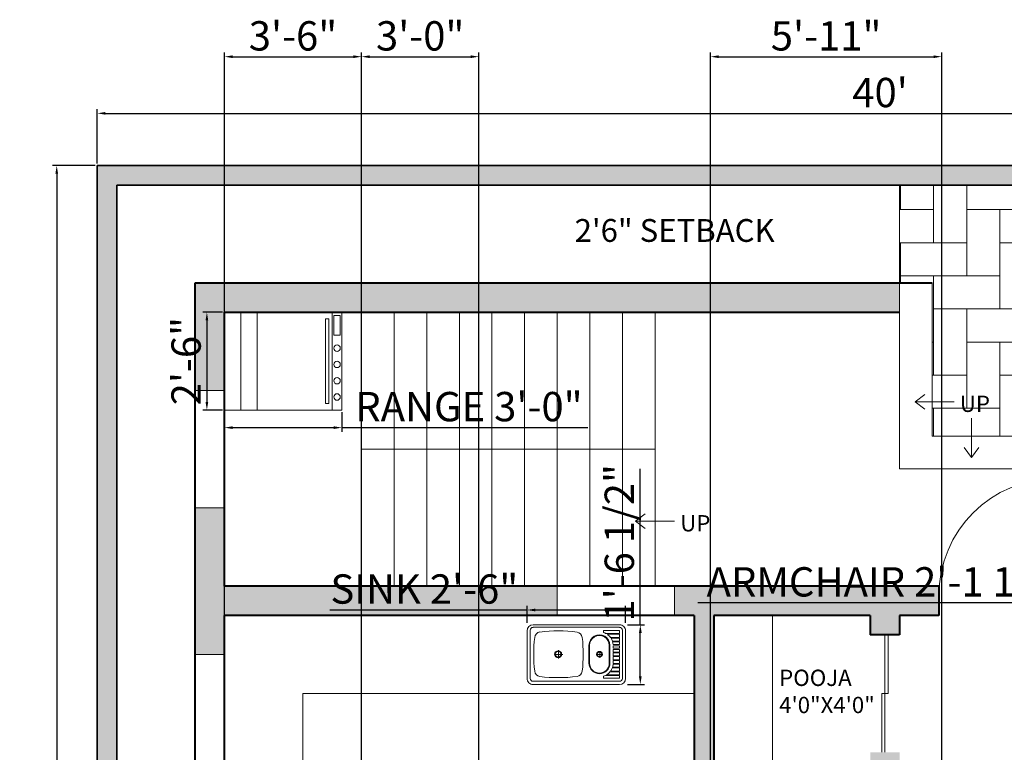
# Model space of a CAD drawing. Units: inches. Extents: x 2337 to 3570, y 1258 to 1938.
# Tile 5 of 30: x 2402 to 2704, y 1713 to 1938. Entities that reach past the tile are written whole.
import ezdxf

# ---------------------------------------------------------------- set-up
doc = ezdxf.new("R2010")
doc.units = ezdxf.units.IN
for name, color, linetype, lineweight in [('A-ANNO-DIMS', 2, 'Continuous', 18), ('A-ANNO-SYMB', 7, 'Continuous', 18), ('A-ANNO-TEXT', 7, 'Continuous', 18), ('A-AREA-IDEN', 7, 'Continuous', 18), ('A-DOOR', 4, 'Continuous', 20), ('A-EQPM', 9, 'Continuous', 18), ('A-FLOR-CASE', 34, 'Continuous', 18), ('A-FLOR-PATT', 252, 'Continuous', 13), ('A-FLOR-STRS', 7, 'Continuous', 20), ('A-GLAZ', 4, 'Continuous', 18), ('A-WALL', 7, 'Continuous', 40), ('C-PROP', 7, 'Continuous', 35), ('Сантехника', 9, 'Continuous', 18)]:
    doc.layers.add(name, color=color, linetype=linetype, lineweight=lineweight)
doc.layers.add('A-WALL-PATT', color=18, linetype='Continuous', lineweight=13, true_color=0x000000)
doc.layers.add('C-PROP-PATT', color=251, linetype='Continuous', lineweight=13, true_color=0x636466)
doc.styles.get("Standard").update_dxf_attribs({"font": 'arial.ttf'})
doc.dimstyles.new('ISO-25', dxfattribs={"dimtxt": 9, "dimasz": 2.5, "dimexe": 1.25, "dimexo": 0.625, "dimtad": 1, "dimdec": 1, "dimlunit": 3, "dimtxsty": 'Standard', "dimcen": 2.5, "dimadec": 0, "dimazin": 0, "dimtfac": 1, "dimtdec": 1, "dimtmove": 0, "dimatfit": 3, "dimfxl": 1, "dimarcsym": 0})

# ---------------------------------------------------------------- blocks, each defined once
blk = doc.blocks.new('*U2')
for p, q in [((0, 0), (0, -6)), ((36, 0), (36, -6))]:
    blk.add_line(p, q)
blk.add_lwpolyline([(0, 0), (0, 36), (1.75, 36), (1.75, 0)], close=True)
blk.add_arc((0, 0), 36, 0, 90)
blk = doc.blocks.new('*D6')
at = {"layer": 'A-ANNO-DIMS', "color": 0, "lineweight": -2, "transparency": 16777216}
for p, q in [((2425.84, 1893.74), (2425.84, 1910.39)), ((2428.34, 1909.14), (2903.34, 1909.14)), ((2905.84, 1893.74), (2905.84, 1910.39))]:
    blk.add_line(p, q, dxfattribs=at)
at = {"layer": 'A-ANNO-DIMS', "color": 0, "transparency": 16777216}
for points in [[(2428.34, 1909.55), (2428.34, 1908.72), (2425.84, 1909.14)], [(2903.34, 1909.55), (2903.34, 1908.72), (2905.84, 1909.14)]]:
    blk.add_solid(points, dxfattribs=at)
at = {"layer": 'Defpoints', "color": 0, "transparency": 16777216}
for p in [(2905.84, 1909.14), (2425.84, 1893.12), (2905.84, 1893.12)]:
    blk.add_point(p, dxfattribs=at)
at = {"layer": 'A-ANNO-DIMS', "color": 0, "transparency": 16777216, "insert": (2665.84, 1914.36), "char_height": 9, "attachment_point": 5}
blk.add_mtext("40'", dxfattribs=at)
blk = doc.blocks.new('*D7')
at = {"layer": 'A-ANNO-DIMS', "color": 0, "lineweight": -2, "transparency": 16777216}
for p, q in [((2425.21, 1893.12), (2412.15, 1893.12)), ((2413.4, 1890.62), (2413.4, 1295.62)), ((2425.21, 1293.12), (2412.15, 1293.12))]:
    blk.add_line(p, q, dxfattribs=at)
at = {"layer": 'A-ANNO-DIMS', "color": 0, "transparency": 16777216}
for points in [[(2412.98, 1890.62), (2413.81, 1890.62), (2413.4, 1893.12)], [(2412.98, 1295.62), (2413.81, 1295.62), (2413.4, 1293.12)]]:
    blk.add_solid(points, dxfattribs=at)
at = {"layer": 'Defpoints', "color": 0, "transparency": 16777216}
for p in [(2425.84, 1893.12), (2413.4, 1293.12), (2425.84, 1293.12)]:
    blk.add_point(p, dxfattribs=at)
at = {"layer": 'A-ANNO-DIMS', "color": 0, "transparency": 16777216, "insert": (2408.18, 1593.12), "char_height": 9, "attachment_point": 5, "rotation": 90}
blk.add_mtext("50'", dxfattribs=at)
blk = doc.blocks.new('sink 1')
for points in [[(5.86, 24.22), (-5.86, 24.22)], [(-7.34, 1.48), (-7.34, 22.73)], [(-6.56, 1.48), (-6.56, 22.73)], [(6.01, 23.43), (-5.86, 23.43)], [(6.72, 1.48), (6.72, 22.73)], [(7.34, 1.48), (7.34, 22.73)], [(0, 15.39), (0, 17.42)], [(1.09, 16.48), (-0.94, 16.48)], [(-2.09, 8.99), (2.28, 8.99)], [(-2.09, 8.84), (2.28, 8.84)], [(0, 5.55), (0, 7.26)], [(-5.78, 5.39), (-5.78, 5.39)], [(-5.31, 5.39), (-5.31, 5.39)], [(-5.16, 4.92), (-5.16, 4.92)], [(0.78, 6.33), (-0.78, 6.33)], [(5.16, 4.92), (5.16, 4.92)], [(5.94, 5.39), (5.94, 5.39)], [(-5, 1.48), (-5, 4.69)], [(-5, 1.48), (-4.22, 1.48), (-4.22, 3.83)], [(-4.84, 4.45), (-4.84, 4.45)], [(-4.22, 3.83), (-4.22, 3.83)], [(-4.06, 1.48), (-4.06, 3.69)], [(-4.06, 1.48), (-3.28, 1.48), (-3.28, 3.27)], [(-3.91, 3.52), (-3.91, 3.52)], [(-3.28, 3.2), (-3.28, 3.2)], [(-3.12, 3.2), (-3.12, 3.2)], [(-2.34, 3.05), (-2.34, 3.05)], [(-2.19, 3.05), (-2.19, 3.05)], [(-2.09, 3.99), (2.28, 3.99)], [(-2.09, 3.84), (2.28, 3.84)], [(-1.41, 3.05), (-1.41, 3.05)], [(-1.25, 3.05), (-1.25, 3.05)], [(-0.47, 1.48), (-1.25, 1.48), (-1.25, 3.05), (-0.47, 3.05)], [(-0.62, 3.05), (-0.62, 3.05)], [(-0.47, 1.48), (-0.47, 3.05)], [(-0.31, 3.05), (-0.31, 3.05)], [(0.47, 1.48), (-0.31, 1.48), (-0.31, 3.05), (0.47, 3.05)], [(0.31, 3.05), (0.31, 3.05)], [(0.47, 1.48), (0.47, 3.05)], [(0.62, 3.05), (0.62, 3.05)], [(1.25, 3.05), (1.25, 3.05)], [(1.56, 3.05), (1.56, 3.05)], [(2.19, 3.05), (2.19, 3.05)], [(2.5, 3.05), (2.5, 3.05)], [(3.12, 3.2), (3.12, 3.2)], [(3.28, 1.48), (4.06, 1.48), (4.06, 3.57)], [(3.28, 1.48), (3.28, 3.2)], [(3.44, 3.2), (3.44, 3.2)], [(4.06, 3.52), (4.06, 3.52)], [(4.22, 1.48), (4.22, 3.67)], [(4.37, 3.83), (4.37, 3.83)], [(5, 4.45), (5, 4.45)], [(6.01, 0.78), (-5.86, 0.78)], [(5.86, 0), (-5.86, 0)], [(-5.78, 1.48), (-5.78, 1.48)], [(-5.16, 1.48), (-5.16, 1.48)], [(-4.84, 1.48), (-4.84, 1.48)], [(-4.22, 1.48), (-4.22, 1.48)], [(-3.91, 1.48), (-3.91, 1.48)], [(-3.28, 1.48), (-3.28, 1.48)], [(-3.12, 1.48), (-3.12, 1.48)], [(-2.34, 1.48), (-2.34, 1.48)], [(-2.19, 1.48), (-2.19, 1.48)], [(-1.41, 1.48), (-1.41, 1.48)], [(-1.25, 1.48), (-1.25, 1.48)], [(-0.62, 1.48), (-0.62, 1.48)], [(-0.31, 1.48), (-0.31, 1.48)], [(0.31, 1.48), (0.31, 1.48)], [(0.62, 1.48), (0.62, 1.48)], [(1.25, 1.48), (1.25, 1.48)], [(1.56, 1.48), (1.56, 1.48)], [(2.19, 1.48), (2.19, 1.48)], [(2.5, 1.48), (2.5, 1.48)], [(3.12, 1.48), (3.12, 1.48)], [(3.44, 1.48), (3.44, 1.48)], [(4.06, 1.48), (4.06, 1.48)], [(4.37, 1.48), (4.37, 1.48)], [(5, 1.48), (5, 1.48)], [(5.16, 1.48), (5.16, 1.48)], [(5.94, 1.48), (5.94, 1.48)]]:
    blk.add_lwpolyline(points)
for points in [[(-5.16, 4.92), (-5.16, 1.48), (-5.78, 1.48), (-5.78, 5.39), (-5.31, 5.39, -0.068511), (-5.16, 4.92)], [(5.16, 4.92, 0.248301), (5.47, 5.39), (5.94, 5.39), (5.94, 1.48), (5.16, 1.48), (5.16, 4.92)], [(4.06, 3.57, -0.061679), (3.32, 3.22)], [(4.22, 1.48), (5, 1.48), (5, 4.45, -0.083542), (4.22, 3.67, -0.083542)]]:
    blk.add_lwpolyline(points, format="xyb")
for points in [[(-3.12, 3.22), (-3.12, 1.48), (-2.34, 1.48), (-2.34, 3.05, -0.06228)], [(2.5, 3.05), (2.5, 1.48), (3.12, 1.48), (3.12, 3.2, -0.050256)]]:
    blk.add_lwpolyline(points, format="xyb", close=True)
for points in [[(-2.19, 3.05), (-1.41, 3.05), (-1.41, 1.48), (-2.19, 1.48)], [(0.62, 3.05), (1.25, 3.05), (1.25, 1.48), (0.62, 1.48)], [(2.19, 1.48), (2.19, 3.05), (1.56, 3.05), (1.56, 1.48)]]:
    blk.add_lwpolyline(points, close=True)
for centre, radius in [((0.09, 16.57), 0.859), ((0.09, 16.57), 0.703), ((0.09, 6.41), 0.703), ((0.09, 6.41), 0.547)]:
    blk.add_circle(centre, radius)
for centre, radius, start, end in [((-5.86, 22.73), 1.48, 90, 180), ((5.86, 22.73), 1.48, 360, 90), ((-5.86, 22.73), 0.703, 90, 180), ((-3.87, 20.82), 1.53, 97.3256, 171.1849), ((0.09, -12.65), 35.23, 83.2159, 96.7841), ((4.06, 20.82), 1.53, 8.8151, 82.6744), ((6.01, 22.73), 0.703, 0, 90), ((30.19, 16.56), 35.85, 172.7947, 187.4213), ((-30, 16.56), 35.85, 352.5787, 7.2053), ((-3.89, 12.12), 1.48, 187.4212, 263.2159), ((0.09, 45.63), 35.23, 263.2159, 276.7841), ((4.08, 12.12), 1.48, 276.7841, 352.5788), ((-2.1, 6.41), 2.58, 90, 270), ((-2.1, 6.41), 2.42, 90, 270), ((2.28, 6.41), 2.58, 270, 90), ((2.28, 6.41), 2.42, 270, 90), ((-2.15, 6.48), 3.36, 212.1095, 232.0862), ((-2.1, 6.41), 3.36, 234.156, 249.3275), ((2.14, 6.36), 3.36, 289.8633, 290.5971), ((-5.86, 1.48), 1.48, 180, 270), ((-5.86, 1.48), 0.703, 180, 270), ((5.86, 1.48), 1.48, 270, 0), ((6.01, 1.48), 0.703, 270, 360)]:
    blk.add_arc(centre, radius, start, end)
blk = doc.blocks.new('Range-Oven - 30 in front')
for p, q in [((0, 33.00005), (30, 33.00005)), ((30, 10), (0, 10)), ((0, 5), (30, 5))]:
    blk.add_line(p, q)
for points in [[(0, 0), (0, 36.00005), (30, 36.00005), (30, 0)], [(1, 33.50005), (1, 35.50005), (7, 35.50005), (7, 33.50005)], [(2, 31.00005), (2, 32.00005), (28, 32.00005), (28, 31.00005)]]:
    blk.add_lwpolyline(points, close=True)
for centre in [(11, 34.50005), (16, 34.50005), (21, 34.50005), (26, 34.50005)]:
    blk.add_circle(centre, 1)
blk = doc.blocks.new('STAIR-UP-ARROW')
for p, q in [((2.25, 12), (2.25, 0)), ((2.25, 0), (0, 3.01)), ((2.25, 0), (4.5, 3.01))]:
    blk.add_line(p, q)
blk = doc.blocks.new('DOOR-SLIDING-36IN')
for p, q in [((1, 36), (1, 0)), ((2, 18), (2, 36)), ((1, 18), (0, 18)), ((0, 18), (0, 0)), ((1, 18), (2, 18))]:
    blk.add_line(p, q)
blk = doc.blocks.new('STAIR-DOUBLE-FLIGHT')
for p, q in [((0, 0), (0, 84)), ((10, 0), (10, 84)), ((20, 0), (20, 84)), ((30, 0), (30, 84)), ((40, 0), (40, 84)), ((50, 0), (50, 84)), ((60, 0), (60, 84)), ((70, 0), (70, 84)), ((80, 0), (80, 84)), ((90, 0), (90, 84)), ((0, 42), (90, 42))]:
    blk.add_line(p, q)
blk = doc.blocks.new('*D80')
at = {"layer": 'A-ANNO-DIMS', "color": 0, "lineweight": -2, "transparency": 16777216}
for p, q in [((2557.6, 1752.87), (2557.6, 1758.02)), ((2587.8, 1752.87), (2587.8, 1758.02)), ((2557.6, 1756.77), (2497.13, 1756.77)), ((2585.3, 1756.77), (2560.1, 1756.77))]:
    blk.add_line(p, q, dxfattribs=at)
at = {"layer": 'A-ANNO-DIMS', "color": 0, "transparency": 16777216}
for points in [[(2560.1, 1757.19), (2560.1, 1756.36), (2557.6, 1756.77)], [(2585.3, 1757.19), (2585.3, 1756.36), (2587.8, 1756.77)]]:
    blk.add_solid(points, dxfattribs=at)
at = {"layer": 'Defpoints', "color": 0, "transparency": 16777216}
for p in [(2557.6, 1756.77), (2557.6, 1752.24), (2587.8, 1752.24)]:
    blk.add_point(p, dxfattribs=at)
at = {"layer": 'A-ANNO-DIMS', "color": 0, "transparency": 16777216, "insert": (2526.11, 1762.05), "char_height": 9, "attachment_point": 5}
blk.add_mtext('SINK 2\'-6"', dxfattribs=at)
blk = doc.blocks.new('*D81')
at = {"layer": 'A-ANNO-DIMS', "color": 0, "lineweight": -2, "transparency": 16777216}
for p, q in [((2592.33, 1752.24), (2592.33, 1800.04)), ((2588.43, 1752.24), (2593.58, 1752.24)), ((2592.33, 1736.42), (2592.33, 1749.74)), ((2588.43, 1733.92), (2593.58, 1733.92))]:
    blk.add_line(p, q, dxfattribs=at)
at = {"layer": 'A-ANNO-DIMS', "color": 0, "transparency": 16777216}
for points in [[(2591.91, 1749.74), (2592.75, 1749.74), (2592.33, 1752.24)], [(2591.91, 1736.42), (2592.75, 1736.42), (2592.33, 1733.92)]]:
    blk.add_solid(points, dxfattribs=at)
at = {"layer": 'Defpoints', "color": 0, "transparency": 16777216}
for p in [(2587.8, 1752.24), (2592.33, 1752.24), (2587.8, 1733.92)]:
    blk.add_point(p, dxfattribs=at)
at = {"layer": 'A-ANNO-DIMS', "color": 0, "transparency": 16777216, "insert": (2587.05, 1777.39), "char_height": 9, "attachment_point": 5, "rotation": 90}
blk.add_mtext('1\'-6 1/2"', dxfattribs=at)
blk = doc.blocks.new('*D88')
at = {"layer": 'A-ANNO-DIMS', "color": 0, "lineweight": -2, "transparency": 16777216}
for p, q in [((2729.73, 1755.74), (2729.73, 1760.22)), ((2755.39, 1755.74), (2755.39, 1760.22)), ((2729.73, 1758.97), (2610.01, 1758.97)), ((2752.89, 1758.97), (2732.23, 1758.97))]:
    blk.add_line(p, q, dxfattribs=at)
at = {"layer": 'A-ANNO-DIMS', "color": 0, "transparency": 16777216}
for points in [[(2732.23, 1759.38), (2732.23, 1758.55), (2729.73, 1758.97)], [(2752.89, 1759.38), (2752.89, 1758.55), (2755.39, 1758.97)]]:
    blk.add_solid(points, dxfattribs=at)
at = {"layer": 'Defpoints', "color": 0, "transparency": 16777216}
for p in [(2729.73, 1758.97), (2729.73, 1755.12), (2755.39, 1755.12)]:
    blk.add_point(p, dxfattribs=at)
at = {"layer": 'A-ANNO-DIMS', "color": 0, "transparency": 16777216, "insert": (2668.62, 1764.24), "char_height": 9, "attachment_point": 5}
blk.add_mtext('ARMCHAIR 2\'-1 1/2"', dxfattribs=at)
blk = doc.blocks.new('*D96')
at = {"layer": 'A-ANNO-DIMS', "color": 0, "lineweight": -2, "transparency": 16777216}
for p, q in [((2464.84, 1817.49), (2464.84, 1811.47)), ((2500.84, 1817.49), (2500.84, 1811.47)), ((2467.34, 1812.72), (2498.34, 1812.72)), ((2500.84, 1812.72), (2576.25, 1812.72))]:
    blk.add_line(p, q, dxfattribs=at)
at = {"layer": 'A-ANNO-DIMS', "color": 0, "transparency": 16777216}
for points in [[(2467.34, 1813.13), (2467.34, 1812.3), (2464.84, 1812.72)], [(2498.34, 1813.13), (2498.34, 1812.3), (2500.84, 1812.72)]]:
    blk.add_solid(points, dxfattribs=at)
at = {"layer": 'Defpoints', "color": 0, "transparency": 16777216}
for p in [(2464.84, 1818.12), (2500.84, 1818.12), (2500.84, 1812.72)]:
    blk.add_point(p, dxfattribs=at)
at = {"layer": 'A-ANNO-DIMS', "color": 0, "transparency": 16777216, "insert": (2539.79, 1818), "char_height": 9, "attachment_point": 5}
blk.add_mtext('RANGE 3\'-0"', dxfattribs=at)
blk = doc.blocks.new('*D97')
at = {"layer": 'A-ANNO-DIMS', "color": 0, "lineweight": -2, "transparency": 16777216}
for p, q in [((2464.21, 1848.12), (2458.19, 1848.12)), ((2459.44, 1845.62), (2459.44, 1820.62)), ((2464.21, 1818.12), (2458.19, 1818.12))]:
    blk.add_line(p, q, dxfattribs=at)
at = {"layer": 'A-ANNO-DIMS', "color": 0, "transparency": 16777216}
for points in [[(2459.02, 1845.62), (2459.85, 1845.62), (2459.44, 1848.12)], [(2459.02, 1820.62), (2459.85, 1820.62), (2459.44, 1818.12)]]:
    blk.add_solid(points, dxfattribs=at)
at = {"layer": 'Defpoints', "color": 0, "transparency": 16777216}
for p in [(2464.84, 1848.12), (2459.44, 1818.12), (2464.84, 1818.12)]:
    blk.add_point(p, dxfattribs=at)
at = {"layer": 'A-ANNO-DIMS', "color": 0, "transparency": 16777216, "insert": (2454.22, 1833.12), "char_height": 9, "attachment_point": 5, "rotation": 90}
blk.add_mtext('2\'-6"', dxfattribs=at)
blk = doc.blocks.new('*D106')
at = {"layer": 'A-ANNO-DIMS', "color": 0, "lineweight": -2, "transparency": 16777216}
for p, q in [((2464.84, 1542.74), (2464.84, 1927.77)), ((2467.34, 1926.52), (2504.34, 1926.52)), ((2506.84, 1542.74), (2506.84, 1927.77))]:
    blk.add_line(p, q, dxfattribs=at)
at = {"layer": 'A-ANNO-DIMS', "color": 0, "transparency": 16777216}
for points in [[(2467.34, 1926.93), (2467.34, 1926.1), (2464.84, 1926.52)], [(2504.34, 1926.93), (2504.34, 1926.1), (2506.84, 1926.52)]]:
    blk.add_solid(points, dxfattribs=at)
at = {"layer": 'Defpoints', "color": 0, "transparency": 16777216}
for p in [(2506.84, 1926.52), (2464.84, 1542.12), (2506.84, 1542.12)]:
    blk.add_point(p, dxfattribs=at)
at = {"layer": 'A-ANNO-DIMS', "color": 0, "transparency": 16777216, "insert": (2485.84, 1931.74), "char_height": 9, "attachment_point": 5}
blk.add_mtext('3\'-6"', dxfattribs=at)
blk = doc.blocks.new('*D107')
at = {"layer": 'A-ANNO-DIMS', "color": 0, "lineweight": -2, "transparency": 16777216}
for p, q in [((2506.84, 1542.74), (2506.84, 1927.77)), ((2509.34, 1926.52), (2540.34, 1926.52)), ((2542.84, 1542.74), (2542.84, 1927.77))]:
    blk.add_line(p, q, dxfattribs=at)
at = {"layer": 'A-ANNO-DIMS', "color": 0, "transparency": 16777216}
for points in [[(2509.34, 1926.93), (2509.34, 1926.1), (2506.84, 1926.52)], [(2540.34, 1926.93), (2540.34, 1926.1), (2542.84, 1926.52)]]:
    blk.add_solid(points, dxfattribs=at)
at = {"layer": 'Defpoints', "color": 0, "transparency": 16777216}
for p in [(2542.84, 1926.52), (2506.84, 1542.12), (2542.84, 1542.12)]:
    blk.add_point(p, dxfattribs=at)
at = {"layer": 'A-ANNO-DIMS', "color": 0, "transparency": 16777216, "insert": (2524.84, 1931.74), "char_height": 9, "attachment_point": 5}
blk.add_mtext('3\'-0"', dxfattribs=at)
blk = doc.blocks.new('*D118')
at = {"layer": 'A-ANNO-DIMS', "color": 0, "lineweight": -2, "transparency": 16777216}
for p, q in [((2613.87, 1497.86), (2613.87, 1927.77)), ((2616.37, 1926.52), (2682.23, 1926.52)), ((2684.73, 1497.86), (2684.73, 1927.77))]:
    blk.add_line(p, q, dxfattribs=at)
at = {"layer": 'A-ANNO-DIMS', "color": 0, "transparency": 16777216}
for points in [[(2616.37, 1926.93), (2616.37, 1926.1), (2613.87, 1926.52)], [(2682.23, 1926.93), (2682.23, 1926.1), (2684.73, 1926.52)]]:
    blk.add_solid(points, dxfattribs=at)
at = {"layer": 'Defpoints', "color": 0, "transparency": 16777216}
for p in [(2684.73, 1926.52), (2613.87, 1497.23), (2684.73, 1497.23)]:
    blk.add_point(p, dxfattribs=at)
at = {"layer": 'A-ANNO-DIMS', "color": 0, "transparency": 16777216, "insert": (2649.3, 1931.74), "char_height": 9, "attachment_point": 5}
blk.add_mtext('5\'-11"', dxfattribs=at)

msp = doc.modelspace()

# ---------------------------------------------------------------- hatches: boundary and pattern name
at = {"layer": 'A-FLOR-PATT', "transparency": 33554687}
h = msp.add_hatch(dxfattribs=at)
h.set_pattern_fill('AR-HBONE', color=256, scale=0.1, angle=45)
h.paths.add_polyline_path([(2902.84, 1875.12), (2899.84, 1875.12), (2899.84, 1887.12), (2671.84, 1887.12), (2671.84, 1857.12), (2681.84, 1857.12), (2681.84, 1810.12), (2719.84, 1810.12), (2719.84, 1764.12), (2872.84, 1764.12), (2899.84, 1764.12), (2899.84, 1779.12), (2902.84, 1779.12)])
h.paths.add_polyline_path([(2854.18, 1832.56), (2857.32, 1832.42), (2861.94, 1831.21, -0.088302), (2868.63, 1828.11), (2871.77, 1825.92, -0.105467), (2873.27, 1824.31), (2874.97, 1823.99), (2877.34, 1822.55), (2875.42, 1827.3), (2873.36, 1826.95, -0.132795), (2873.22, 1833.51), (2876.1, 1833.32), (2876.1, 1832.97), (2877.28, 1832.48, -0.091085), (2878.86, 1831.44, -0.069602), (2881.45, 1828.18, -0.141553), (2886.25, 1809.41, -0.141553), (2881.49, 1790.63, -0.069602), (2878.91, 1787.37, -0.091085), (2877.32, 1786.33), (2876.14, 1785.83, -0.354729), (2875.73, 1785.45), (2873.27, 1785.29, -0.132795), (2873.39, 1791.84), (2875.45, 1791.49), (2877.36, 1796.25), (2874.99, 1794.81), (2873.3, 1794.48, -0.105467), (2871.8, 1792.87), (2868.67, 1790.67, -0.088302), (2861.99, 1787.56), (2857.37, 1786.34), (2854.23, 1786.2), (2827.8, 1783.01, -0.315912), (2819.63, 1782.95), (2793.54, 1785.74), (2798.79, 1786.94), (2825.85, 1785.28, 0.026512), (2832.53, 1785.23), (2857.37, 1786.34), (2861.99, 1787.56, 0.088302), (2868.67, 1790.67), (2871.8, 1792.87, 0.191215), (2873.93, 1796.11), (2875.79, 1805.13, 0.102572), (2875.78, 1813.67), (2873.91, 1822.68, 0.191215), (2871.77, 1825.92), (2868.63, 1828.11, 0.088302), (2861.94, 1831.21), (2857.32, 1832.42), (2832.48, 1833.49, 0.026512), (2825.8, 1833.42), (2798.75, 1831.7), (2793.5, 1832.9), (2819.58, 1835.73, -0.315912), (2827.75, 1835.69)], flags=16)
h.paths.add_polyline_path([(2862.34, 1826.57), (2867.3, 1826, -0.316515), (2870.31, 1823.31), (2872.44, 1814.15, -0.11452), (2872.45, 1804.64), (2870.34, 1795.48, -0.316515), (2867.33, 1792.79), (2862.37, 1792.2, -0.464922), (2861.4, 1793.12), (2861.86, 1801.97), (2861.84, 1809.39), (2861.85, 1816.81), (2861.36, 1825.65, -0.464922)], flags=16)
h.paths.add_polyline_path([(2821.29, 1791.09), (2807.57, 1791.5, -0.405226), (2805.02, 1794.12), (2805.02, 1794.12, 0.40508), (2807.57, 1791.5), (2821.29, 1791.09, 0.423258), (2824, 1793.72), (2824, 1793.72, -0.423258)], flags=16)
h.paths.add_polyline_path([(2879.43, 1814.8), (2881.74, 1813.82), (2882.58, 1811.67), (2882.72, 1809.41), (2882.59, 1807.14), (2881.75, 1804.99), (2879.44, 1804.01), (2880.04, 1807.7, 0.081616), (2880.04, 1811.11)], flags=0)
h.paths.add_polyline_path([(2796.96, 1829.72), (2796.14, 1815.43, 0.029076), (2796.15, 1803.21), (2797, 1788.93, -0.409057), (2796.19, 1788), (2791.05, 1787.61), (2785.76, 1792.94, -0.173254), (2784.26, 1796.14), (2783.47, 1804.33, -0.047466), (2783.46, 1814.29), (2784.23, 1822.48, -0.173254), (2785.73, 1825.69), (2791.01, 1831.02), (2796.15, 1830.64, -0.409057)], flags=16)
h.paths.add_polyline_path([(2750.34, 1835.79), (2750.01, 1834.37, 0.040009), (2748.77, 1826.06), (2748.63, 1824.02), (2750.53, 1825.24), (2756.61, 1827.24), (2771.95, 1829.42), (2781.4, 1831.05), (2780.1, 1822.89), (2779.44, 1814.33), (2779.14, 1809.3), (2779.45, 1804.28), (2780.13, 1795.72), (2781.44, 1787.56), (2771.99, 1789.17), (2756.65, 1791.34), (2750.56, 1793.32), (2748.66, 1794.54), (2748.8, 1792.49, 0.040009), (2750.06, 1784.19), (2750.4, 1782.77), (2745.9, 1784.64), (2744.1, 1788.13), (2743.1, 1791.92), (2741.07, 1803), (2740.86, 1809.27), (2741.06, 1815.55), (2743.06, 1826.62), (2744.06, 1830.42), (2745.85, 1833.91)], flags=16)
h.paths.add_polyline_path([(2761.18, 1831.2), (2754.85, 1829.51), (2754.56, 1830.83, -0.143032), (2754.62, 1831.81), (2755.05, 1833), (2761.17, 1831.71, -0.789416)], flags=16)
h.paths.add_polyline_path([(2761.23, 1787.38), (2754.89, 1789.06), (2754.6, 1787.74, 0.143032), (2754.66, 1786.76), (2755.1, 1785.57), (2761.21, 1786.87, 0.789416)], flags=16)
h.paths.add_polyline_path([(2689.03, 1816.17), (2701.27, 1816.17), (2701.27, 1823.8), (2689.03, 1823.8)], flags=24)
h.paths.add_polyline_path([(2755.38, 1858.95), (2808.72, 1858.95), (2808.72, 1885.07), (2755.38, 1885.07)], flags=24)
at = {"layer": 'A-WALL-PATT'}
h = msp.add_hatch(color=256, dxfattribs=at)
h.dxf.hatch_style = 1
h.paths.add_polyline_path([(2671.84, 1857.12), (2455.84, 1857.12), (2455.84, 1824.12), (2464.84, 1824.12), (2464.84, 1848.12), (2671.84, 1848.12)])
h.paths.add_polyline_path([(2566.84, 1764.12), (2464.84, 1764.12), (2464.84, 1788.12), (2455.84, 1788.12), (2455.84, 1743.12), (2464.84, 1743.12), (2464.84, 1755.12), (2566.84, 1755.12)])
h.paths.add_polyline_path([(2683.84, 1761.12), (2683.84, 1764.12), (2602.84, 1764.12), (2602.84, 1755.12), (2608.84, 1755.12), (2608.84, 1701.12), (2662.84, 1701.12), (2662.84, 1605.12), (2671.84, 1605.12), (2671.84, 1713.12), (2662.84, 1713.12), (2662.84, 1707.12), (2614.84, 1707.12), (2614.84, 1755.12), (2662.84, 1755.12), (2662.84, 1749.12), (2671.84, 1749.12), (2671.84, 1755.12), (2683.84, 1755.12)])
h.paths.add_polyline_path([(2464.84, 1707.12), (2455.84, 1707.12), (2455.84, 1617.12), (2464.84, 1617.12), (2464.84, 1635.12), (2506.84, 1635.12), (2506.84, 1641.12), (2464.84, 1641.12)])
h.paths.add_polyline_path([(2542.84, 1551.12), (2464.84, 1551.12), (2464.84, 1569.12), (2455.84, 1569.12), (2455.84, 1518.12), (2464.84, 1518.12), (2464.84, 1542.12), (2542.84, 1542.12)])
h.paths.add_polyline_path([(2464.84, 1482.12), (2455.84, 1482.12), (2455.84, 1410.12), (2464.84, 1410.12)])
h.paths.add_polyline_path([(2626.84, 1350.12), (2590.84, 1350.12), (2590.84, 1380.12), (2584.84, 1380.12), (2584.84, 1350.12), (2464.84, 1350.12), (2464.84, 1374.12), (2455.84, 1374.12), (2455.84, 1341.12), (2626.84, 1341.12)])
h.paths.add_polyline_path([(2662.84, 1416.12), (2686.84, 1416.12), (2686.84, 1422.12), (2590.84, 1422.12), (2590.84, 1542.12), (2680.84, 1542.12), (2680.84, 1551.12), (2671.84, 1551.12), (2671.84, 1557.12), (2662.84, 1557.12), (2662.84, 1551.12), (2578.84, 1551.12), (2578.84, 1542.12), (2584.84, 1542.12), (2584.84, 1410.12), (2590.84, 1410.12), (2590.84, 1416.12), (2656.84, 1416.12), (2656.84, 1350.12), (2650.84, 1350.12), (2650.84, 1341.12), (2731.84, 1341.12), (2731.84, 1362.12), (2722.84, 1362.12), (2722.84, 1350.12), (2662.84, 1350.12)])
h.paths.add_polyline_path([(2731.84, 1434.12), (2722.84, 1434.12), (2722.84, 1422.12), (2716.84, 1422.12), (2716.84, 1416.12), (2722.84, 1416.12), (2722.84, 1386.12), (2731.84, 1386.12)], flags=17)
h.paths.add_polyline_path([(2731.84, 1542.12), (2752.84, 1542.12), (2752.84, 1551.12), (2716.84, 1551.12), (2716.84, 1545.12), (2716.84, 1542.12), (2722.84, 1542.12), (2722.84, 1482.12), (2731.84, 1482.12)])
h.paths.add_polyline_path([(2809.84, 1551.12), (2788.84, 1551.12), (2788.84, 1542.12), (2809.84, 1542.12), (2809.84, 1548.12)])
h.paths.add_polyline_path([(2872.84, 1647.12), (2863.84, 1647.12), (2863.84, 1551.12), (2857.84, 1551.12), (2857.84, 1548.12), (2857.84, 1542.12), (2872.84, 1542.12)])
h.paths.add_polyline_path([(2872.84, 1764.12), (2827.84, 1764.12), (2827.84, 1755.12), (2863.84, 1755.12), (2863.84, 1719.12), (2872.84, 1719.12)])
h.paths.add_polyline_path([(2755.84, 1764.12), (2719.84, 1764.12), (2719.84, 1755.12), (2755.84, 1755.12)])
at = {"layer": 'C-PROP-PATT'}
h = msp.add_hatch(color=256, dxfattribs=at)
h.dxf.hatch_style = 1
h.paths.add_polyline_path([(2905.84, 1893.12), (2425.84, 1893.12), (2425.84, 1293.12), (2731.84, 1293.12), (2731.84, 1299.12), (2431.84, 1299.12), (2431.84, 1887.12), (2899.84, 1887.12), (2899.84, 1875.12), (2905.84, 1875.12)])
h.paths.add_polyline_path([(2845.84, 1299.12), (2827.84, 1299.12), (2827.84, 1293.12), (2845.84, 1293.12)], flags=17)
h.paths.add_polyline_path([(2905.84, 1779.12), (2899.84, 1779.12), (2899.84, 1299.12), (2893.84, 1299.12), (2893.84, 1293.12), (2905.84, 1293.12)], flags=17)

# ---------------------------------------------------------------- linework, layer by layer
at = {"layer": 'A-FLOR-CASE'}
for p, q in [((2632.84, 1755.12), (2632.84, 1707.12)), ((2608.84, 1731.12), (2488.84, 1731.12)), ((2488.84, 1641.12), (2488.84, 1731.12))]:
    msp.add_line(p, q, dxfattribs=at)
at = {"layer": 'A-FLOR-STRS'}
for p, q in [((2671.84, 1887.12), (2671.84, 1800.12)), ((2681.84, 1857.12), (2681.84, 1810.12)), ((2719.84, 1810.12), (2681.84, 1810.12)), ((2719.84, 1800.12), (2671.84, 1800.12))]:
    msp.add_line(p, q, dxfattribs=at)
at = {"layer": 'A-GLAZ'}
for p, q in [((2464.84, 1824.12), (2455.84, 1824.12)), ((2464.84, 1788.12), (2455.84, 1788.12)), ((2566.84, 1764.12), (2566.84, 1755.12)), ((2602.84, 1764.12), (2602.84, 1755.12)), ((2464.84, 1743.12), (2455.84, 1743.12))]:
    msp.add_line(p, q, dxfattribs=at)
at = {"layer": 'A-WALL'}
for p, q in [((2455.84, 1857.12), (2681.84, 1857.12)), ((2455.84, 1341.12), (2455.84, 1857.12)), ((2464.84, 1848.12), (2671.84, 1848.12)), ((2464.84, 1764.12), (2464.84, 1848.12)), ((2683.84, 1764.12), (2464.84, 1764.12)), ((2683.84, 1764.12), (2683.84, 1755.12)), ((2608.84, 1755.12), (2464.84, 1755.12)), ((2464.84, 1641.12), (2464.84, 1755.12)), ((2608.84, 1755.12), (2608.84, 1683.12)), ((2614.84, 1755.12), (2614.84, 1707.12)), ((2662.84, 1755.12), (2614.84, 1755.12)), ((2662.84, 1755.12), (2662.84, 1749.12)), ((2671.84, 1755.12), (2671.84, 1749.12)), ((2683.84, 1755.12), (2671.84, 1755.12)), ((2671.84, 1749.12), (2662.84, 1749.12))]:
    msp.add_line(p, q, dxfattribs=at)
at = {"layer": 'C-PROP'}
for p, q in [((2425.84, 1893.12), (2905.84, 1893.12)), ((2425.84, 1293.12), (2425.84, 1893.12)), ((2431.84, 1299.12), (2431.84, 1887.12)), ((2431.84, 1887.12), (2899.84, 1887.12))]:
    msp.add_line(p, q, dxfattribs=at)

# ---------------------------------------------------------------- block references
at = {"layer": 'A-ANNO-SYMB'}
for p, rotation in [((2676.57, 1822.89), 270.0000000000029), ((2590.84, 1786.25), 270.0000000000043)]:
    msp.add_blockref('STAIR-UP-ARROW', p, dxfattribs=dict(at, rotation=rotation))
msp.add_blockref('STAIR-UP-ARROW', (2691.6, 1803.6), dxfattribs=at)
at = {"layer": 'A-DOOR', "xscale": -1}
msp.add_blockref('*U2', (2719.84, 1761.12), dxfattribs=at)
at = {"layer": 'A-DOOR'}
msp.add_blockref('DOOR-SLIDING-36IN', (2666.34, 1713.12), dxfattribs=at)
at = {"layer": 'A-EQPM', "rotation": 270}
msp.add_blockref('Range-Oven - 30 in front', (2464.84, 1848.12), dxfattribs=at)
at = {"layer": 'A-FLOR-STRS'}
msp.add_blockref('STAIR-DOUBLE-FLIGHT', (2506.84, 1764.12), dxfattribs=at)
at = {"layer": 'Сантехника', "xscale": 1.24732326381372, "yscale": 1.24732326381372, "zscale": 1.24732326381372, "rotation": 89.99999999999999}
msp.add_blockref('sink 1', (2587.8, 1743.08), dxfattribs=at)

# ---------------------------------------------------------------- texts
at = {"layer": 'A-ANNO-TEXT'}
for p in [(2690.3, 1817.53), (2604.57, 1780.88)]:
    msp.add_text('UP', height=5, dxfattribs=at).set_placement(p)
at = {"layer": 'A-ANNO-TEXT', "insert": (2572.21, 1876.71), "char_height": 7, "attachment_point": 1}
msp.add_mtext_dynamic_manual_height_columns('2\'6" SETBACK', width=66.911, gutter_width=12.5, heights=[0], dxfattribs=at)
at = {"layer": 'A-AREA-IDEN', "insert": (2634.9, 1738.47), "char_height": 5, "attachment_point": 1}
msp.add_mtext_dynamic_manual_height_columns('POOJA\\P4\'0"X4\'0"', width=66.911, gutter_width=12.5, heights=[0], dxfattribs=at)

# ---------------------------------------------------------------- dimensions: what is measured, and where the dimension line sits
at = {"layer": 'A-ANNO-DIMS'}
for base, p1, p2, override, picture, middle in [((2506.84, 1926.52), (2464.84, 1542.12), (2506.84, 1542.12), {"dimdec": 1, "dimlfac": 1, "dimrnd": 0, "dimzin": 1, "dimdsep": 46, "dimlunit": 4, "dimfrac": 2}, '*D106', (2485.84, 1931.74)), ((2542.84, 1926.52), (2506.84, 1542.12), (2542.84, 1542.12), {"dimdec": 1, "dimlfac": 1, "dimrnd": 0, "dimzin": 1, "dimdsep": 46, "dimlunit": 4, "dimfrac": 2}, '*D107', (2524.84, 1931.74)), ((2684.73, 1926.52), (2613.87, 1497.23), (2684.73, 1497.23), {"dimdec": 1, "dimlfac": 1, "dimrnd": 0, "dimzin": 1, "dimdsep": 46, "dimlunit": 4, "dimfrac": 2}, '*D118', (2649.3, 1931.74)), ((2905.84, 1909.14), (2425.84, 1893.12), (2905.84, 1893.12), {"dimclrd": 0, "dimclre": 0, "dimclrt": 0}, '*D6', (2665.84, 1914.36))]:
    dim = msp.add_linear_dim(base=base, p1=p1, p2=p2, dimstyle='ISO-25', override=override, dxfattribs=at)
    dim.commit()
    dim.dimension.update_dxf_attribs({"geometry": picture, "text_midpoint": middle})
for base, p1, p2, angle, override, picture, middle in [((2413.4, 1293.12), (2425.84, 1893.12), (2425.84, 1293.12), 90, {"dimclrd": 0, "dimclre": 0, "dimclrt": 0}, '*D7', (2408.18, 1593.12)), ((2459.44, 1818.12), (2464.84, 1848.12), (2464.84, 1818.12), 270, {"dimdec": 1, "dimlfac": 1, "dimrnd": 0, "dimzin": 1, "dimdsep": 46, "dimlunit": 4, "dimfrac": 2}, '*D97', (2454.22, 1833.12)), ((2592.33, 1752.24), (2587.8, 1733.92), (2587.8, 1752.24), 90, {"dimdec": 1, "dimlfac": 1, "dimrnd": 0, "dimzin": 1, "dimdsep": 46, "dimlunit": 4, "dimfrac": 2}, '*D81', (2587.05, 1777.39))]:
    dim = msp.add_linear_dim(base=base, p1=p1, p2=p2, angle=angle, dimstyle='ISO-25', override=override, dxfattribs=at)
    dim.commit()
    dim.dimension.update_dxf_attribs({"geometry": picture, "text_midpoint": middle})
dim = msp.add_linear_dim(base=(2500.84, 1812.72), p1=(2464.84, 1818.12), p2=(2500.84, 1818.12), text='RANGE <>', dimstyle='ISO-25', override={"dimdec": 1, "dimlfac": 1, "dimrnd": 0, "dimzin": 1, "dimdsep": 46, "dimlunit": 4, "dimfrac": 2}, dxfattribs=at)
dim.commit()
dim.dimension.update_dxf_attribs({"geometry": '*D96', "text_midpoint": (2539.79, 1818)})
for base, p1, p2, text, picture, middle in [((2729.73, 1758.97), (2755.39, 1755.12), (2729.73, 1755.12), 'ARMCHAIR <>', '*D88', (2668.62, 1764.24)), ((2557.6, 1756.77), (2587.8, 1752.24), (2557.6, 1752.24), 'SINK <>', '*D80', (2526.11, 1762.05))]:
    dim = msp.add_linear_dim(base=base, p1=p1, p2=p2, angle=180, text=text, dimstyle='ISO-25', override={"dimdec": 1, "dimlfac": 1, "dimrnd": 0, "dimzin": 1, "dimdsep": 46, "dimlunit": 4, "dimfrac": 2}, dxfattribs=at)
    dim.commit()
    dim.dimension.update_dxf_attribs({"geometry": picture, "text_midpoint": middle})

doc.saveas('drawing.dxf')
